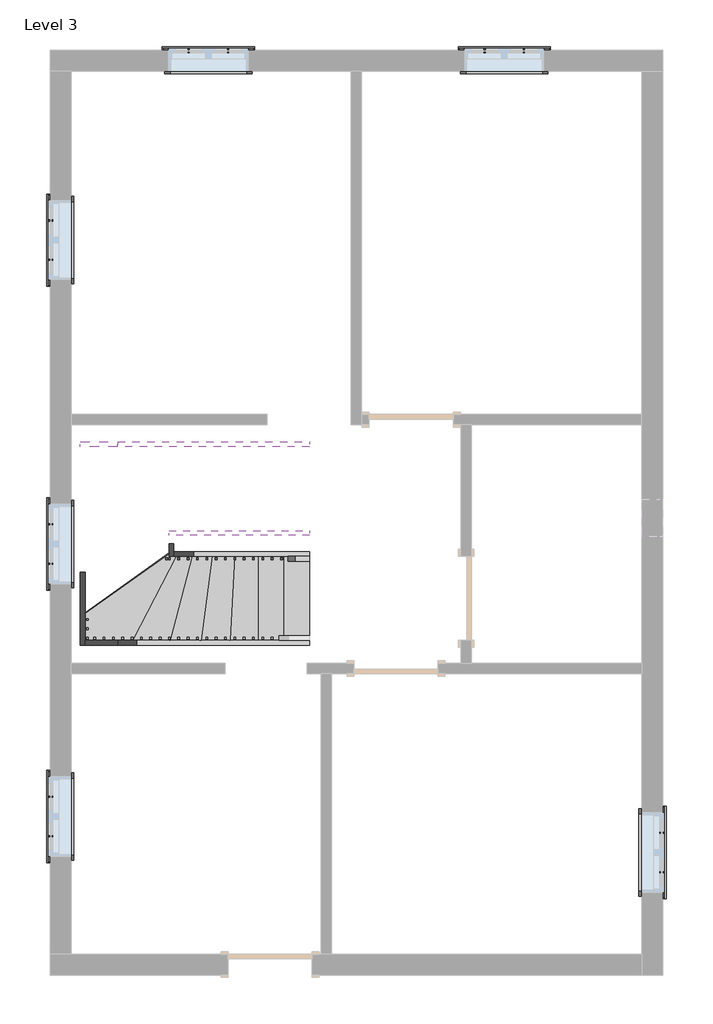
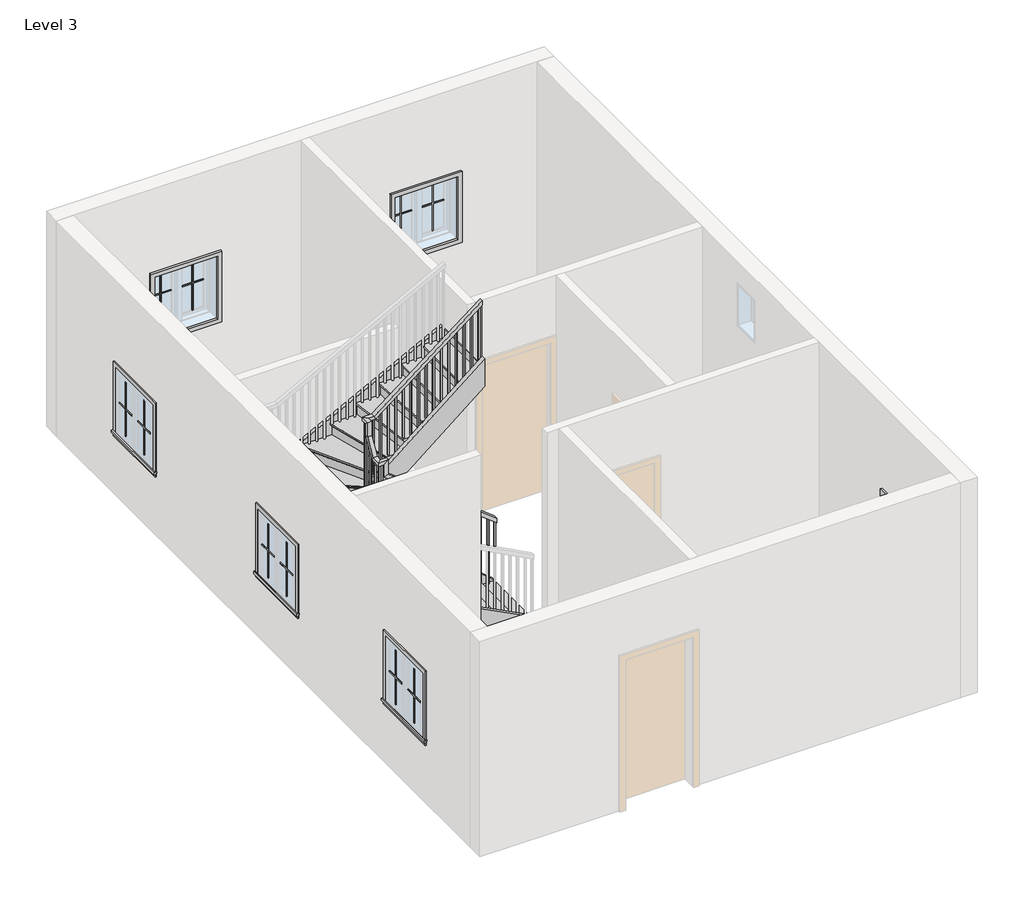
# One storey, part 2 of 2: 24 proxies, 8 members, 1 railing, 1 stair flight.
"""IFC4 building model written with IfcOpenShell, lengths in millimetres."""

from ifc_helpers import new_model, si_unit, frame, origin, place, context, project, spatial, polyline, outline, extrude, faceted_brep, transform, mapped, element, save
from components import muntin_pattern_2x2_muntin_pattern_2x2_b3fe6957, muntin_pattern_2x2_muntin_pattern_2x2_3e0ecaf2, trim_window_exterior_flat_with_sill_41619996, trim_window_interior_flat_picture_frame_51c85655, stair_flight_e257120f

model = new_model("IFC4")

# Units and contexts
model_context = context("Model", 3, world=origin())
ifc_project = project(units=[si_unit("LENGTHUNIT", "METRE", prefix="MILLI")], contexts=[model_context])

# Site, building, storey
site = spatial("IfcSite", under=ifc_project)
building = spatial("IfcBuilding", under=site)
storey = spatial("IfcBuildingStorey", under=building, Name="Level 3", Elevation=3200.4)

# Proxies
placement = place(None, origin())
muntin_pattern_2x2_muntin_pattern_2x2_shape = muntin_pattern_2x2_muntin_pattern_2x2_b3fe6957(model_context)
element("IfcBuildingElementProxy", 1, Name="Muntin Pattern_2x2 : Muntin Pattern_2x2", ObjectType="Muntin Pattern_2x2 : Muntin Pattern_2x2", at=placement, inside=storey, context=model_context, shape_type="MappedRepresentation", body=[
    mapped(muntin_pattern_2x2_muntin_pattern_2x2_shape, transform((-3096.8324167, 5150.2179147, 4184.65), x_axis=(1.0, 0.0, 0.0), y_axis=(0.0, 1.0, 0.0), z_axis=(0.0, 0.0, 1.0))),
])
element("IfcBuildingElementProxy", 2, Name="Muntin Pattern_2x2 : Muntin Pattern_2x2", ObjectType="Muntin Pattern_2x2 : Muntin Pattern_2x2", at=placement, inside=storey, context=model_context, shape_type="MappedRepresentation", body=[
    mapped(muntin_pattern_2x2_muntin_pattern_2x2_shape, transform((122.6175833, 5150.2179147, 4184.65), x_axis=(1.0, 0.0, 0.0), y_axis=(0.0, 1.0, 0.0), z_axis=(0.0, 0.0, 1.0))),
])
element("IfcBuildingElementProxy", 3, Name="Muntin Pattern_2x2 : Muntin Pattern_2x2", ObjectType="Muntin Pattern_2x2 : Muntin Pattern_2x2", at=placement, inside=storey, context=model_context, shape_type="MappedRepresentation", body=[
    mapped(muntin_pattern_2x2_muntin_pattern_2x2_shape, transform((2051.4300833, -3350.8445853, 4184.65), x_axis=(0.0, -1.0, 0.0), y_axis=(1.0, 0.0, 0.0), z_axis=(0.0, 0.0, 1.0))),
])
element("IfcBuildingElementProxy", 4, Name="Muntin Pattern_2x2 : Muntin Pattern_2x2", ObjectType="Muntin Pattern_2x2 : Muntin Pattern_2x2", at=placement, inside=storey, context=model_context, shape_type="MappedRepresentation", body=[
    mapped(muntin_pattern_2x2_muntin_pattern_2x2_shape, transform((-4597.0199167, -426.6695853, 4184.65), x_axis=(0.0, 1.0, 0.0), y_axis=(-1.0, 0.0, 0.0), z_axis=(0.0, 0.0, 1.0))),
])
element("IfcBuildingElementProxy", 5, Name="Muntin Pattern_2x2 : Muntin Pattern_2x2", ObjectType="Muntin Pattern_2x2 : Muntin Pattern_2x2", at=placement, inside=storey, context=model_context, shape_type="MappedRepresentation", body=[
    mapped(muntin_pattern_2x2_muntin_pattern_2x2_shape, transform((-4597.0199167, -3388.9445853, 4184.65), x_axis=(0.0, 1.0, 0.0), y_axis=(-1.0, 0.0, 0.0), z_axis=(0.0, 0.0, 1.0))),
])
element("IfcBuildingElementProxy", 6, Name="Muntin Pattern_2x2 : Muntin Pattern_2x2", ObjectType="Muntin Pattern_2x2 : Muntin Pattern_2x2", at=placement, inside=storey, context=model_context, shape_type="MappedRepresentation", body=[
    mapped(muntin_pattern_2x2_muntin_pattern_2x2_shape, transform((-4597.0199167, 2878.5054147, 4184.65), x_axis=(0.0, 1.0, 0.0), y_axis=(-1.0, 0.0, 0.0), z_axis=(0.0, 0.0, 1.0))),
])
muntin_pattern_2x2_muntin_pattern_2x2_2_shape = muntin_pattern_2x2_muntin_pattern_2x2_3e0ecaf2(model_context)
element("IfcBuildingElementProxy", 7, Name="Muntin Pattern_2x2 : Muntin Pattern_2x2", ObjectType="Muntin Pattern_2x2 : Muntin Pattern_2x2", at=placement, inside=storey, context=model_context, shape_type="MappedRepresentation", body=[
    mapped(muntin_pattern_2x2_muntin_pattern_2x2_2_shape, transform((-2668.2074167, 5150.2179147, 4184.65), x_axis=(-1.0, 0.0, 0.0), y_axis=(0.0, -1.0, 0.0), z_axis=(0.0, 0.0, 1.0))),
])
element("IfcBuildingElementProxy", 8, Name="Muntin Pattern_2x2 : Muntin Pattern_2x2", ObjectType="Muntin Pattern_2x2 : Muntin Pattern_2x2", at=placement, inside=storey, context=model_context, shape_type="MappedRepresentation", body=[
    mapped(muntin_pattern_2x2_muntin_pattern_2x2_2_shape, transform((551.2425833, 5150.2179147, 4184.65), x_axis=(-1.0, 0.0, 0.0), y_axis=(0.0, -1.0, 0.0), z_axis=(0.0, 0.0, 1.0))),
])
element("IfcBuildingElementProxy", 9, Name="Muntin Pattern_2x2 : Muntin Pattern_2x2", ObjectType="Muntin Pattern_2x2 : Muntin Pattern_2x2", at=placement, inside=storey, context=model_context, shape_type="MappedRepresentation", body=[
    mapped(muntin_pattern_2x2_muntin_pattern_2x2_2_shape, transform((2051.4300833, -3779.4695853, 4184.65), x_axis=(0.0, 1.0, 0.0), y_axis=(-1.0, 0.0, 0.0), z_axis=(0.0, 0.0, 1.0))),
])
element("IfcBuildingElementProxy", 10, Name="Muntin Pattern_2x2 : Muntin Pattern_2x2", ObjectType="Muntin Pattern_2x2 : Muntin Pattern_2x2", at=placement, inside=storey, context=model_context, shape_type="MappedRepresentation", body=[
    mapped(muntin_pattern_2x2_muntin_pattern_2x2_2_shape, transform((-4597.0199167, 1.9554147, 4184.65), x_axis=(0.0, -1.0, 0.0), y_axis=(1.0, 0.0, 0.0), z_axis=(0.0, 0.0, 1.0))),
])
element("IfcBuildingElementProxy", 11, Name="Muntin Pattern_2x2 : Muntin Pattern_2x2", ObjectType="Muntin Pattern_2x2 : Muntin Pattern_2x2", at=placement, inside=storey, context=model_context, shape_type="MappedRepresentation", body=[
    mapped(muntin_pattern_2x2_muntin_pattern_2x2_2_shape, transform((-4597.0199167, -2960.3195853, 4184.65), x_axis=(0.0, -1.0, 0.0), y_axis=(1.0, 0.0, 0.0), z_axis=(0.0, 0.0, 1.0))),
])
element("IfcBuildingElementProxy", 12, Name="Muntin Pattern_2x2 : Muntin Pattern_2x2", ObjectType="Muntin Pattern_2x2 : Muntin Pattern_2x2", at=placement, inside=storey, context=model_context, shape_type="MappedRepresentation", body=[
    mapped(muntin_pattern_2x2_muntin_pattern_2x2_2_shape, transform((-4597.0199167, 3307.1304147, 4184.65), x_axis=(0.0, -1.0, 0.0), y_axis=(1.0, 0.0, 0.0), z_axis=(0.0, 0.0, 1.0))),
])
trim_window_exterior_flat_with_sill_shape = trim_window_exterior_flat_with_sill_41619996(model_context)
element("IfcBuildingElementProxy", 13, Name="Trim-Window-Exterior-Flat : with Sill", ObjectType="Trim-Window-Exterior-Flat : with Sill", at=placement, inside=storey, context=model_context, shape_type="MappedRepresentation", body=[
    mapped(trim_window_exterior_flat_with_sill_shape, transform((-2882.5199167, 5159.7429147, 5029.2), x_axis=(-1.0, 0.0, 0.0), y_axis=(0.0, 0.0, 1.0), z_axis=(0.0, 1.0, 0.0))),
])
element("IfcBuildingElementProxy", 14, Name="Trim-Window-Exterior-Flat : with Sill", ObjectType="Trim-Window-Exterior-Flat : with Sill", at=placement, inside=storey, context=model_context, shape_type="MappedRepresentation", body=[
    mapped(trim_window_exterior_flat_with_sill_shape, transform((336.9300833, 5159.7429147, 5029.2), x_axis=(-1.0, 0.0, 0.0), y_axis=(0.0, 0.0, 1.0), z_axis=(0.0, 1.0, 0.0))),
])
element("IfcBuildingElementProxy", 15, Name="Trim-Window-Exterior-Flat : with Sill", ObjectType="Trim-Window-Exterior-Flat : with Sill", at=placement, inside=storey, context=model_context, shape_type="MappedRepresentation", body=[
    mapped(trim_window_exterior_flat_with_sill_shape, transform((2060.9550833, -3565.1570853, 5029.2), x_axis=(0.0, 1.0, 0.0), y_axis=(0.0, 0.0, 1.0), z_axis=(1.0, 0.0, 0.0))),
])
element("IfcBuildingElementProxy", 16, Name="Trim-Window-Exterior-Flat : with Sill", ObjectType="Trim-Window-Exterior-Flat : with Sill", at=placement, inside=storey, context=model_context, shape_type="MappedRepresentation", body=[
    mapped(trim_window_exterior_flat_with_sill_shape, transform((-4606.5449167, -212.3570853, 5029.2), x_axis=(0.0, -1.0, 0.0), y_axis=(0.0, 0.0, 1.0), z_axis=(-1.0, 0.0, 0.0))),
])
element("IfcBuildingElementProxy", 17, Name="Trim-Window-Exterior-Flat : with Sill", ObjectType="Trim-Window-Exterior-Flat : with Sill", at=placement, inside=storey, context=model_context, shape_type="MappedRepresentation", body=[
    mapped(trim_window_exterior_flat_with_sill_shape, transform((-4606.5449167, -3174.6320853, 5029.2), x_axis=(0.0, -1.0, 0.0), y_axis=(0.0, 0.0, 1.0), z_axis=(-1.0, 0.0, 0.0))),
])
element("IfcBuildingElementProxy", 18, Name="Trim-Window-Exterior-Flat : with Sill", ObjectType="Trim-Window-Exterior-Flat : with Sill", at=placement, inside=storey, context=model_context, shape_type="MappedRepresentation", body=[
    mapped(trim_window_exterior_flat_with_sill_shape, transform((-4606.5449167, 3092.8179147, 5029.2), x_axis=(0.0, -1.0, 0.0), y_axis=(0.0, 0.0, 1.0), z_axis=(-1.0, 0.0, 0.0))),
])
trim_window_interior_flat_picture_frame_shape = trim_window_interior_flat_picture_frame_51c85655(model_context)
element("IfcBuildingElementProxy", 19, Name="Trim-Window-Interior-Flat : Picture Frame", ObjectType="Trim-Window-Interior-Flat : Picture Frame", at=placement, inside=storey, context=model_context, shape_type="MappedRepresentation", body=[
    mapped(trim_window_interior_flat_picture_frame_shape, transform((-2882.5199167, 4931.1429147, 5029.2), x_axis=(1.0, 0.0, 0.0), y_axis=(0.0, 0.0, 1.0), z_axis=(0.0, -1.0, 0.0))),
])
element("IfcBuildingElementProxy", 20, Name="Trim-Window-Interior-Flat : Picture Frame", ObjectType="Trim-Window-Interior-Flat : Picture Frame", at=placement, inside=storey, context=model_context, shape_type="MappedRepresentation", body=[
    mapped(trim_window_interior_flat_picture_frame_shape, transform((336.9300833, 4931.1429147, 5029.2), x_axis=(1.0, 0.0, 0.0), y_axis=(0.0, 0.0, 1.0), z_axis=(0.0, -1.0, 0.0))),
])
element("IfcBuildingElementProxy", 21, Name="Trim-Window-Interior-Flat : Picture Frame", ObjectType="Trim-Window-Interior-Flat : Picture Frame", at=placement, inside=storey, context=model_context, shape_type="MappedRepresentation", body=[
    mapped(trim_window_interior_flat_picture_frame_shape, transform((1832.3550833, -3565.1570853, 5029.2), x_axis=(0.0, -1.0, 0.0), y_axis=(0.0, 0.0, 1.0), z_axis=(-1.0, 0.0, 0.0))),
])
element("IfcBuildingElementProxy", 22, Name="Trim-Window-Interior-Flat : Picture Frame", ObjectType="Trim-Window-Interior-Flat : Picture Frame", at=placement, inside=storey, context=model_context, shape_type="MappedRepresentation", body=[
    mapped(trim_window_interior_flat_picture_frame_shape, transform((-4377.9449167, -212.3570853, 5029.2), x_axis=(0.0, 1.0, 0.0), y_axis=(0.0, 0.0, 1.0), z_axis=(1.0, 0.0, 0.0))),
])
element("IfcBuildingElementProxy", 23, Name="Trim-Window-Interior-Flat : Picture Frame", ObjectType="Trim-Window-Interior-Flat : Picture Frame", at=placement, inside=storey, context=model_context, shape_type="MappedRepresentation", body=[
    mapped(trim_window_interior_flat_picture_frame_shape, transform((-4377.9449167, -3174.6320853, 5029.2), x_axis=(0.0, 1.0, 0.0), y_axis=(0.0, 0.0, 1.0), z_axis=(1.0, 0.0, 0.0))),
])
element("IfcBuildingElementProxy", 24, Name="Trim-Window-Interior-Flat : Picture Frame", ObjectType="Trim-Window-Interior-Flat : Picture Frame", at=placement, inside=storey, context=model_context, shape_type="MappedRepresentation", body=[
    mapped(trim_window_interior_flat_picture_frame_shape, transform((-4377.9449167, 3092.8179147, 5029.2), x_axis=(0.0, 1.0, 0.0), y_axis=(0.0, 0.0, 1.0), z_axis=(1.0, 0.0, 0.0))),
])

# Members
element("IfcMember", 25, ObjectType="Stringer - 2\" Width", at=placement, inside=storey, context=model_context, shape_type="SweptSolid", body=[
    extrude(outline(polyline([(3200.4, -1783.4132248), (3430.039954, -1783.4132248), (4505.7956453, -3870.8304165), (4162.900629, -3870.8304165), (3200.4, -2003.1755424), (3200.4, -1783.4132248)])), frame((0.0, -1310.9070853, 0.0), z_axis=(0.0, 1.0, 0.0), x_axis=(0.0, 0.0, 1.0)), (0.0, 0.0, 1.0), 50.8),
])
element("IfcMember", 26, ObjectType="Stringer - 2\" Width", at=placement, inside=storey, context=model_context, shape_type="SweptSolid", body=[
    extrude(outline(polyline([(-3870.8304165, -1260.1070853), (-3870.8304165, -1310.9070853), (-4225.5449167, -1310.9070853), (-4225.5449167, -1260.1070853), (-3870.8304165, -1260.1070853)])), frame((0.0, 0.0, 4162.900629), z_axis=(0.0, 0.0, 1.0), x_axis=(1.0, 0.0, 0.0)), (0.0, 0.0, 1.0), 342.8950162),
])
element("IfcMember", 27, ObjectType="Stringer - 2\" Width", at=placement, inside=storey, context=model_context, shape_type="SweptSolid", body=[
    extrude(outline(polyline([(-1310.9070853, 4200.9956453), (-1310.9070853, 4489.4952212), (811.1127974, 5170.3972697), (848.0929147, 5170.3972697), (848.0929147, 4839.3682298), (-1141.3846024, 4200.9956453), (-1310.9070853, 4200.9956453)])), frame((-4276.3449167, 0.0, 0.0), z_axis=(1.0, 0.0, 0.0), x_axis=(0.0, 1.0, 0.0)), (0.0, 0.0, 1.0), 50.8),
])
element("IfcMember", 28, ObjectType="Stringer - 2\" Width", at=placement, inside=storey, context=model_context, shape_type="SweptSolid", body=[
    extrude(outline(polyline([(-4276.3449167, 848.0929147), (-4276.3449167, 898.8929147), (-3870.8304165, 898.8929147), (-3870.8304165, 848.0929147), (-4276.3449167, 848.0929147)])), frame((0.0, 0.0, 4850.2904473), z_axis=(0.0, 0.0, 1.0), x_axis=(1.0, 0.0, 0.0)), (0.0, 0.0, 1.0), 320.1068224),
])
element("IfcMember", 29, ObjectType="Stringer - 2\" Width", at=placement, inside=storey, context=model_context, shape_type="SweptSolid", body=[
    extrude(outline(polyline([(5170.3972697, -3870.8304165), (4850.2904473, -3870.8304165), (5926.0461385, -1783.4132248), (6246.1529609, -1783.4132248), (5170.3972697, -3870.8304165)])), frame((0.0, 848.0929147, 0.0), z_axis=(0.0, 1.0, 0.0), x_axis=(0.0, 0.0, 1.0)), (0.0, 0.0, 1.0), 50.8),
])
element("IfcMember", 30, ObjectType="Stringer - 2\" Width", at=placement, inside=storey, context=model_context, shape_type="SweptSolid", body=[
    extrude(outline(polyline([(3200.4, -1783.4132248), (3376.5764461, -1783.4132248), (4580.818648, -3260.3449167), (4187.5410923, -3260.3449167), (3200.4, -2049.6748694), (3200.4, -1783.4132248)])), frame((0.0, -345.7070853, 0.0), z_axis=(0.0, 1.0, 0.0), x_axis=(0.0, 0.0, 1.0)), (0.0, 0.0, 1.0), 50.8),
])
element("IfcMember", 31, ObjectType="Stringer - 2\" Width", at=placement, inside=storey, context=model_context, shape_type="SweptSolid", body=[
    extrude(outline(polyline([(-345.7070853, 4228.9617647), (-345.7070853, 4773.6682978), (-139.0699679, 5126.5409689), (-117.1070853, 5126.5409689), (-117.1070853, 4560.865107), (-311.464868, 4228.9617647), (-345.7070853, 4228.9617647)])), frame((-3311.1449167, 0.0, 0.0), z_axis=(1.0, 0.0, 0.0), x_axis=(0.0, 1.0, 0.0)), (0.0, 0.0, 1.0), 50.8),
])
element("IfcMember", 32, ObjectType="Stringer - 2\" Width", at=placement, inside=storey, context=model_context, shape_type="SweptSolid", body=[
    extrude(outline(polyline([(5126.5409689, -3311.1449167), (4733.2634131, -3311.1449167), (5978.9262875, -1783.4132248), (6372.2038432, -1783.4132248), (5126.5409689, -3311.1449167)])), frame((0.0, -117.1070853, 0.0), z_axis=(0.0, 1.0, 0.0), x_axis=(0.0, 0.0, 1.0)), (0.0, 0.0, 1.0), 50.8),
])

# Railing
element("IfcRailing", 33, ObjectType="Handrail - Rectangular", at=placement, inside=storey, context=model_context, shape_type="SolidModel", body=[
    faceted_brep([(-1783.4132248, -396.5070853, 4284.1333333), (-1783.4132248, -396.5070853, 4219.8000346), (-1783.4132248, -345.7070853, 4219.8000346), (-1783.4132248, -345.7070853, 4284.1333333), (-3234.9449167, -396.5070853, 5412.0191036), (-3285.7449167, -396.5070853, 5387.1590024), (-3285.7449167, -345.7070853, 5387.1590024), (-3234.9449167, -345.7070853, 5412.0191036), (-3234.9449167, -396.5070853, 5615.0281882), (-3285.7449167, -396.5070853, 5564.2281882), (-3285.7449167, -345.7070853, 5564.2281882), (-3234.9449167, -345.7070853, 5615.0281882), (-3361.9449167, -396.5070853, 5615.0281882), (-3361.9449167, -396.5070853, 5564.2281882), (-3311.1449167, -345.7070853, 5564.2281882), (-3311.1449167, -345.7070853, 5615.0281882), (-3361.9449167, -269.5070853, 5615.0281882), (-3361.9449167, -240.3857515, 5564.2281882), (-3311.1449167, -240.3857515, 5564.2281882), (-3311.1449167, -269.5070853, 5615.0281882), (-3361.9449167, -142.5070853, 5831.9051451), (-3361.9449167, -91.7070853, 5818.1256424), (-3311.1449167, -91.7070853, 5818.1256424), (-3311.1449167, -142.5070853, 5831.9051451), (-3361.9449167, -142.5070853, 6034.9142297), (-3361.9449167, -91.7070853, 5984.1142297), (-3311.1449167, -91.7070853, 5984.1142297), (-3311.1449167, -142.5070853, 6034.9142297), (-3361.9449167, -15.5070853, 6034.9142297), (-3361.9449167, -15.5070853, 5984.1142297), (-3311.1449167, -66.3070853, 5984.1142297), (-3311.1449167, -66.3070853, 6034.9142297), (-3234.9449167, -15.5070853, 6034.9142297), (-3217.5282487, -15.5070853, 5984.1142297), (-3217.5282487, -66.3070853, 5984.1142297), (-3234.9449167, -66.3070853, 6034.9142297), (-1783.4132248, -15.5070853, 7162.8), (-1783.4132248, -66.3070853, 7162.8), (-1783.4132248, -66.3070853, 7098.4667013), (-1783.4132248, -15.5070853, 7098.4667013)], [[[0, 1, 2, 3]], [[1, 0, 4, 5]], [[2, 1, 5, 6]], [[3, 2, 6, 7]], [[0, 3, 7, 4]], [[5, 4, 8, 9]], [[6, 5, 9, 10]], [[7, 6, 10, 11]], [[4, 7, 11, 8]], [[9, 8, 12, 13]], [[10, 9, 13, 14]], [[11, 10, 14, 15]], [[8, 11, 15, 12]], [[13, 12, 16, 17]], [[14, 13, 17, 18]], [[15, 14, 18, 19]], [[12, 15, 19, 16]], [[17, 16, 20, 21]], [[18, 17, 21, 22]], [[19, 18, 22, 23]], [[16, 19, 23, 20]], [[21, 20, 24, 25]], [[22, 21, 25, 26]], [[23, 22, 26, 27]], [[20, 23, 27, 24]], [[25, 24, 28, 29]], [[26, 25, 29, 30]], [[27, 26, 30, 31]], [[24, 27, 31, 28]], [[29, 28, 32, 33]], [[30, 29, 33, 34]], [[31, 30, 34, 35]], [[28, 31, 35, 32]], [[36, 37, 38, 39]], [[33, 32, 36, 39]], [[34, 33, 39, 38]], [[35, 34, 38, 37]], [[32, 35, 37, 36]]]),
    extrude(outline(polyline([(7083.2316852, -1803.0199167), (7068.4292361, -1822.0699167), (6079.0666667, -1822.0699167), (6079.0666667, -1803.0199167), (7083.2316852, -1803.0199167)])), frame((0.0, -50.4320853, 0.0), z_axis=(0.0, 1.0, 0.0), x_axis=(0.0, 0.0, 1.0)), (0.0, 0.0, 1.0), 19.05),
    extrude(outline(polyline([(7004.2852902, -1904.6199167), (6989.4828411, -1923.6699167), (6079.0666667, -1923.6699167), (6079.0666667, -1904.6199167), (7004.2852902, -1904.6199167)])), frame((0.0, -50.4320853, 0.0), z_axis=(0.0, 1.0, 0.0), x_axis=(0.0, 0.0, 1.0)), (0.0, 0.0, 1.0), 19.05),
    extrude(outline(polyline([(6925.3388952, -2006.2199167), (6910.5364462, -2025.2699167), (6079.0666667, -2025.2699167), (6079.0666667, -2006.2199167), (6925.3388952, -2006.2199167)])), frame((0.0, -50.4320853, 0.0), z_axis=(0.0, 1.0, 0.0), x_axis=(0.0, 0.0, 1.0)), (0.0, 0.0, 1.0), 19.05),
    extrude(outline(polyline([(6846.3925003, -2107.8199167), (6831.5900512, -2126.8699167), (5909.7333333, -2126.8699167), (5909.7333333, -2107.8199167), (6846.3925003, -2107.8199167)])), frame((0.0, -50.4320853, 0.0), z_axis=(0.0, 1.0, 0.0), x_axis=(0.0, 0.0, 1.0)), (0.0, 0.0, 1.0), 19.05),
    extrude(outline(polyline([(6767.4461053, -2209.4199167), (6752.6436562, -2228.4699167), (5909.7333333, -2228.4699167), (5909.7333333, -2209.4199167), (6767.4461053, -2209.4199167)])), frame((0.0, -50.4320853, 0.0), z_axis=(0.0, 1.0, 0.0), x_axis=(0.0, 0.0, 1.0)), (0.0, 0.0, 1.0), 19.05),
    extrude(outline(polyline([(6688.4997103, -2311.0199167), (6673.6972613, -2330.0699167), (5909.7333333, -2330.0699167), (5909.7333333, -2311.0199167), (6688.4997103, -2311.0199167)])), frame((0.0, -50.4320853, 0.0), z_axis=(0.0, 1.0, 0.0), x_axis=(0.0, 0.0, 1.0)), (0.0, 0.0, 1.0), 19.05),
    extrude(outline(polyline([(6609.5533154, -2412.6199167), (6594.7508663, -2431.6699167), (5740.4, -2431.6699167), (5740.4, -2412.6199167), (6609.5533154, -2412.6199167)])), frame((0.0, -50.4320853, 0.0), z_axis=(0.0, 1.0, 0.0), x_axis=(0.0, 0.0, 1.0)), (0.0, 0.0, 1.0), 19.05),
    extrude(outline(polyline([(6530.6069204, -2514.2199167), (6515.8044713, -2533.2699167), (5740.4, -2533.2699167), (5740.4, -2514.2199167), (6530.6069204, -2514.2199167)])), frame((0.0, -50.4320853, 0.0), z_axis=(0.0, 1.0, 0.0), x_axis=(0.0, 0.0, 1.0)), (0.0, 0.0, 1.0), 19.05),
    extrude(outline(polyline([(6451.6605254, -2615.8199167), (6436.8580764, -2634.8699167), (5571.0666667, -2634.8699167), (5571.0666667, -2615.8199167), (6451.6605254, -2615.8199167)])), frame((0.0, -50.4320853, 0.0), z_axis=(0.0, 1.0, 0.0), x_axis=(0.0, 0.0, 1.0)), (0.0, 0.0, 1.0), 19.05),
    extrude(outline(polyline([(6372.7141304, -2717.4199167), (6357.9116814, -2736.4699167), (5571.0666667, -2736.4699167), (5571.0666667, -2717.4199167), (6372.7141304, -2717.4199167)])), frame((0.0, -50.4320853, 0.0), z_axis=(0.0, 1.0, 0.0), x_axis=(0.0, 0.0, 1.0)), (0.0, 0.0, 1.0), 19.05),
    extrude(outline(polyline([(6293.7677355, -2819.0199167), (6278.9652864, -2838.0699167), (5571.0666667, -2838.0699167), (5571.0666667, -2819.0199167), (6293.7677355, -2819.0199167)])), frame((0.0, -50.4320853, 0.0), z_axis=(0.0, 1.0, 0.0), x_axis=(0.0, 0.0, 1.0)), (0.0, 0.0, 1.0), 19.05),
    extrude(outline(polyline([(6214.8213405, -2920.6199167), (6200.0188914, -2939.6699167), (5401.7333333, -2939.6699167), (5401.7333333, -2920.6199167), (6214.8213405, -2920.6199167)])), frame((0.0, -50.4320853, 0.0), z_axis=(0.0, 1.0, 0.0), x_axis=(0.0, 0.0, 1.0)), (0.0, 0.0, 1.0), 19.05),
    extrude(outline(polyline([(6135.8749455, -3022.2199167), (6121.0724965, -3041.2699167), (5401.7333333, -3041.2699167), (5401.7333333, -3022.2199167), (6135.8749455, -3022.2199167)])), frame((0.0, -50.4320853, 0.0), z_axis=(0.0, 1.0, 0.0), x_axis=(0.0, 0.0, 1.0)), (0.0, 0.0, 1.0), 19.05),
    extrude(outline(polyline([(6056.9285506, -3123.8199167), (6042.1261015, -3142.8699167), (5232.4, -3142.8699167), (5232.4, -3123.8199167), (6056.9285506, -3123.8199167)])), frame((0.0, -50.4320853, 0.0), z_axis=(0.0, 1.0, 0.0), x_axis=(0.0, 0.0, 1.0)), (0.0, 0.0, 1.0), 19.05),
    extrude(outline(polyline([(5977.9821556, -3225.4199167), (5963.1797065, -3244.4699167), (5232.4, -3244.4699167), (5232.4, -3225.4199167), (5977.9821556, -3225.4199167)])), frame((0.0, -50.4320853, 0.0), z_axis=(0.0, 1.0, 0.0), x_axis=(0.0, 0.0, 1.0)), (0.0, 0.0, 1.0), 19.05),
    extrude(outline(polyline([(-3327.0199167, -75.8320853), (-3346.0699167, -75.8320853), (-3346.0699167, -56.7820853), (-3327.0199167, -56.7820853), (-3327.0199167, -75.8320853)])), frame((0.0, 0.0, 4893.7333333), z_axis=(0.0, 0.0, 1.0), x_axis=(1.0, 0.0, 0.0)), (0.0, 0.0, 1.0), 1090.3808964),
    extrude(outline(polyline([(-177.4320853, 5671.7336964), (-158.3820853, 5704.26524), (-158.3820853, 4724.4), (-177.4320853, 4724.4), (-177.4320853, 5671.7336964)])), frame((-3346.0699167, 0.0, 0.0), z_axis=(1.0, 0.0, 0.0), x_axis=(0.0, 1.0, 0.0)), (0.0, 0.0, 1.0), 19.05),
    extrude(outline(polyline([(-279.0320853, 5498.2321309), (-259.9820853, 5530.7636744), (-259.9820853, 4555.0666667), (-279.0320853, 4555.0666667), (-279.0320853, 5498.2321309)])), frame((-3346.0699167, 0.0, 0.0), z_axis=(1.0, 0.0, 0.0), x_axis=(0.0, 1.0, 0.0)), (0.0, 0.0, 1.0), 19.05),
    extrude(outline(polyline([(-3297.8882248, -361.5820853), (-3297.8882248, -380.6320853), (-3316.9382248, -380.6320853), (-3316.9382248, -361.5820853), (-3297.8882248, -361.5820853)])), frame((0.0, 0.0, 4385.7333333), z_axis=(0.0, 0.0, 1.0), x_axis=(1.0, 0.0, 0.0)), (0.0, 0.0, 1.0), 1178.4948549),
    extrude(outline(polyline([(5317.6483397, -3196.2882248), (5332.4507888, -3215.3382248), (4216.4, -3215.3382248), (4216.4, -3196.2882248), (5317.6483397, -3196.2882248)])), frame((0.0, -380.6320853, 0.0), z_axis=(0.0, 1.0, 0.0), x_axis=(0.0, 0.0, 1.0)), (0.0, 0.0, 1.0), 19.05),
    extrude(outline(polyline([(5238.7019447, -3094.6882248), (5253.5043938, -3113.7382248), (4216.4, -3113.7382248), (4216.4, -3094.6882248), (5238.7019447, -3094.6882248)])), frame((0.0, -380.6320853, 0.0), z_axis=(0.0, 1.0, 0.0), x_axis=(0.0, 0.0, 1.0)), (0.0, 0.0, 1.0), 19.05),
    extrude(outline(polyline([(5159.7555498, -2993.0882248), (5174.5579988, -3012.1382248), (4047.0666667, -3012.1382248), (4047.0666667, -2993.0882248), (5159.7555498, -2993.0882248)])), frame((0.0, -380.6320853, 0.0), z_axis=(0.0, 1.0, 0.0), x_axis=(0.0, 0.0, 1.0)), (0.0, 0.0, 1.0), 19.05),
    extrude(outline(polyline([(5080.8091548, -2891.4882248), (5095.6116039, -2910.5382248), (4047.0666667, -2910.5382248), (4047.0666667, -2891.4882248), (5080.8091548, -2891.4882248)])), frame((0.0, -380.6320853, 0.0), z_axis=(0.0, 1.0, 0.0), x_axis=(0.0, 0.0, 1.0)), (0.0, 0.0, 1.0), 19.05),
    extrude(outline(polyline([(5001.8627598, -2789.8882248), (5016.6652089, -2808.9382248), (3877.7333333, -2808.9382248), (3877.7333333, -2789.8882248), (5001.8627598, -2789.8882248)])), frame((0.0, -380.6320853, 0.0), z_axis=(0.0, 1.0, 0.0), x_axis=(0.0, 0.0, 1.0)), (0.0, 0.0, 1.0), 19.05),
    extrude(outline(polyline([(4922.9163649, -2688.2882248), (4937.7188139, -2707.3382248), (3877.7333333, -2707.3382248), (3877.7333333, -2688.2882248), (4922.9163649, -2688.2882248)])), frame((0.0, -380.6320853, 0.0), z_axis=(0.0, 1.0, 0.0), x_axis=(0.0, 0.0, 1.0)), (0.0, 0.0, 1.0), 19.05),
    extrude(outline(polyline([(4843.9699699, -2586.6882248), (4858.7724189, -2605.7382248), (3708.4, -2605.7382248), (3708.4, -2586.6882248), (4843.9699699, -2586.6882248)])), frame((0.0, -380.6320853, 0.0), z_axis=(0.0, 1.0, 0.0), x_axis=(0.0, 0.0, 1.0)), (0.0, 0.0, 1.0), 19.05),
    extrude(outline(polyline([(4765.0235749, -2485.0882248), (4779.826024, -2504.1382248), (3708.4, -2504.1382248), (3708.4, -2485.0882248), (4765.0235749, -2485.0882248)])), frame((0.0, -380.6320853, 0.0), z_axis=(0.0, 1.0, 0.0), x_axis=(0.0, 0.0, 1.0)), (0.0, 0.0, 1.0), 19.05),
    extrude(outline(polyline([(4686.0771799, -2383.4882248), (4700.879629, -2402.5382248), (3708.4, -2402.5382248), (3708.4, -2383.4882248), (4686.0771799, -2383.4882248)])), frame((0.0, -380.6320853, 0.0), z_axis=(0.0, 1.0, 0.0), x_axis=(0.0, 0.0, 1.0)), (0.0, 0.0, 1.0), 19.05),
    extrude(outline(polyline([(4607.130785, -2281.8882248), (4621.933234, -2300.9382248), (3539.0666667, -2300.9382248), (3539.0666667, -2281.8882248), (4607.130785, -2281.8882248)])), frame((0.0, -380.6320853, 0.0), z_axis=(0.0, 1.0, 0.0), x_axis=(0.0, 0.0, 1.0)), (0.0, 0.0, 1.0), 19.05),
    extrude(outline(polyline([(4528.18439, -2180.2882248), (4542.9868391, -2199.3382248), (3539.0666667, -2199.3382248), (3539.0666667, -2180.2882248), (4528.18439, -2180.2882248)])), frame((0.0, -380.6320853, 0.0), z_axis=(0.0, 1.0, 0.0), x_axis=(0.0, 0.0, 1.0)), (0.0, 0.0, 1.0), 19.05),
    extrude(outline(polyline([(4449.237995, -2078.6882248), (4464.0404441, -2097.7382248), (3539.0666667, -2097.7382248), (3539.0666667, -2078.6882248), (4449.237995, -2078.6882248)])), frame((0.0, -380.6320853, 0.0), z_axis=(0.0, 1.0, 0.0), x_axis=(0.0, 0.0, 1.0)), (0.0, 0.0, 1.0), 19.05),
    extrude(outline(polyline([(4370.2916001, -1977.0882248), (4385.0940491, -1996.1382248), (3369.7333333, -1996.1382248), (3369.7333333, -1977.0882248), (4370.2916001, -1977.0882248)])), frame((0.0, -380.6320853, 0.0), z_axis=(0.0, 1.0, 0.0), x_axis=(0.0, 0.0, 1.0)), (0.0, 0.0, 1.0), 19.05),
    extrude(outline(polyline([(4291.3452051, -1875.4882248), (4306.1476541, -1894.5382248), (3369.7333333, -1894.5382248), (3369.7333333, -1875.4882248), (4291.3452051, -1875.4882248)])), frame((0.0, -380.6320853, 0.0), z_axis=(0.0, 1.0, 0.0), x_axis=(0.0, 0.0, 1.0)), (0.0, 0.0, 1.0), 19.05),
    extrude(outline(polyline([(-3327.0199167, -50.4320853), (-3346.0699167, -50.4320853), (-3346.0699167, -31.3820853), (-3327.0199167, -31.3820853), (-3327.0199167, -50.4320853)])), frame((0.0, 0.0, 5063.0666667), z_axis=(0.0, 0.0, 1.0), x_axis=(1.0, 0.0, 0.0)), (0.0, 0.0, 1.0), 921.0475631),
    extrude(outline(polyline([(-3327.0199167, -361.5820853), (-3327.0199167, -380.6320853), (-3346.0699167, -380.6320853), (-3346.0699167, -361.5820853), (-3327.0199167, -361.5820853)])), frame((0.0, 0.0, 4385.7333333), z_axis=(0.0, 0.0, 1.0), x_axis=(1.0, 0.0, 0.0)), (0.0, 0.0, 1.0), 1178.4948549),
    extrude(outline(polyline([(7098.4667013, -1783.4132248), (7083.6642523, -1802.4632248), (6079.0666667, -1802.4632248), (6079.0666667, -1783.4132248), (7098.4667013, -1783.4132248)])), frame((0.0, -50.4320853, 0.0), z_axis=(0.0, 1.0, 0.0), x_axis=(0.0, 0.0, 1.0)), (0.0, 0.0, 1.0), 19.05),
    extrude(outline(polyline([(4219.8000346, -1783.4132248), (4234.6024837, -1802.4632248), (3369.7333333, -1802.4632248), (3369.7333333, -1783.4132248), (4219.8000346, -1783.4132248)])), frame((0.0, -380.6320853, 0.0), z_axis=(0.0, 1.0, 0.0), x_axis=(0.0, 0.0, 1.0)), (0.0, 0.0, 1.0), 19.05),
])

# Stair flight
stair_flight_shape = stair_flight_e257120f(model_context)
element("IfcStairFlight", 34, ObjectType="2\" Tread 1\" Nosing 1/4\" Riser", at=placement, inside=storey, context=model_context, shape_type="MappedRepresentation", body=[
    mapped(stair_flight_shape, transform((0.0, 0.0, 0.0), x_axis=(1.0, 0.0, 0.0), y_axis=(0.0, 1.0, 0.0), z_axis=(0.0, 0.0, 1.0))),
])

save(model, "model.ifc")

# Revit data of these elements
# Type "Muntin Pattern_2x2 : Muntin Pattern_2x2"
#   Width [instance default] = 4' - 0"
#   Thickness = 0' - 0 1/2"
#   Height [instance default] = 4' - 0"
#   Distance = 0' - 0 3/4"
#   Interior Material [instance default] = none
#   Exterior Material [instance default] = none
#   Default Elevation = 0
# Type "Trim-Window-Exterior-Flat : with Sill"
#   Trim Width = 0' - 2 1/4"
#   Trim Thickness_Picture Frame = 0' - 1 1/4"
#   Trim Thickness_with Sill = 0' - 0 3/4"
#   Sill Thickness = 0' - 1 1/4"
#   Opening Width [instance default] = 2' - 0"
#   Opening Height [instance default] = 3' - 0"
#   Default Elevation = 4' - 0"
#   Sill = yes
#   Picture Frame = no
#   Trim Material [instance default] = none
# Type "Trim-Window-Interior-Flat : Picture Frame"
#   Trim Thickness_Picture Frame = 0' - 1 1/4"
#   Trim Width = 0' - 2 1/4"
#   Trim Thickness_with Sill = 0' - 0 3/4"
#   Sill Thickness = 0' - 1 1/4"
#   Opening Width [instance default] = 2' - 0"
#   Opening Height [instance default] = 3' - 0"
#   Default Elevation = 4' - 0"
#   Sill = no
#   Picture Frame = yes
#   Trim Material [instance default] = none
# Type "Handrail - Rectangular"
#   Assembly Code = "C2010400"
#   built-in parameter 1008612 = 0.0416667 (stored number, unit not read)
#   built-in parameter 1008611 = 0.0416667 (stored number, unit not read)
#   built-in parameter 1008609 = 0.333333 (stored number, unit not read)
#   built-in parameter 1008604 = 0.166667 (stored number, unit not read)
#   built-in parameter 1008603 = 0.166667 (stored number, unit not read)
#   Railing Height = 3' - 0"
#   built-in parameter 1008630 = 2
#   built-in parameter 1008610 = 2
#   built-in parameter 1008618 = Baluster - Square : 3/4"
# Elements 1, 2, 3, 4, 5, 6, 7, 8, 9, 10, 11, 12 (IfcBuildingElementProxy, "Muntin Pattern_2x2 : Muntin Pattern_2x2")
#   Width = 0' - 11 5/8"
#   Height = 2' - 6 1/2"
#   Interior Material = Wood - Stained
#   Exterior Material = Clad - White
#   Phase Created = New Construction
#   Materials on its faces: "Clad - White", "Wood - Stained"
# Elements 13, 14, 15, 16, 17, 18 (IfcBuildingElementProxy, "Trim-Window-Exterior-Flat : with Sill")
#   Opening Width = 2' - 10"
#   Opening Height = 3' - 0"
#   Trim Material = Clad - White
#   Phase Created = New Construction
#   Materials on its faces: "Clad - White"
# Elements 19, 20, 21, 22, 23, 24 (IfcBuildingElementProxy, "Trim-Window-Interior-Flat : Picture Frame")
#   Opening Width = 2' - 10"
#   Opening Height = 3' - 0"
#   Trim Material = Wood - Stained
#   Phase Created = New Construction
#   Materials on its faces: "Wood - Stained"
# Elements 25, 26, 27, 28, 29, 30, 31, 32 (IfcMember, "Stringer - 2\" Width")
#   Phase Created = New Construction
# Element 33 (IfcRailing, "Handrail - Rectangular")
#   Phase Created = New Construction
# Element 34 (IfcStairFlight, "2\" Tread 1\" Nosing 1/4\" Riser")
#   Phase Created = New Construction
# Materials
#   "Clad - White": class "Wood", colour RGB 242 242 238, transparency 0, Cost = 0
#   "Wood - Stained": class "Wood", colour RGB 224 178 126, transparency 0, Cost = 0
